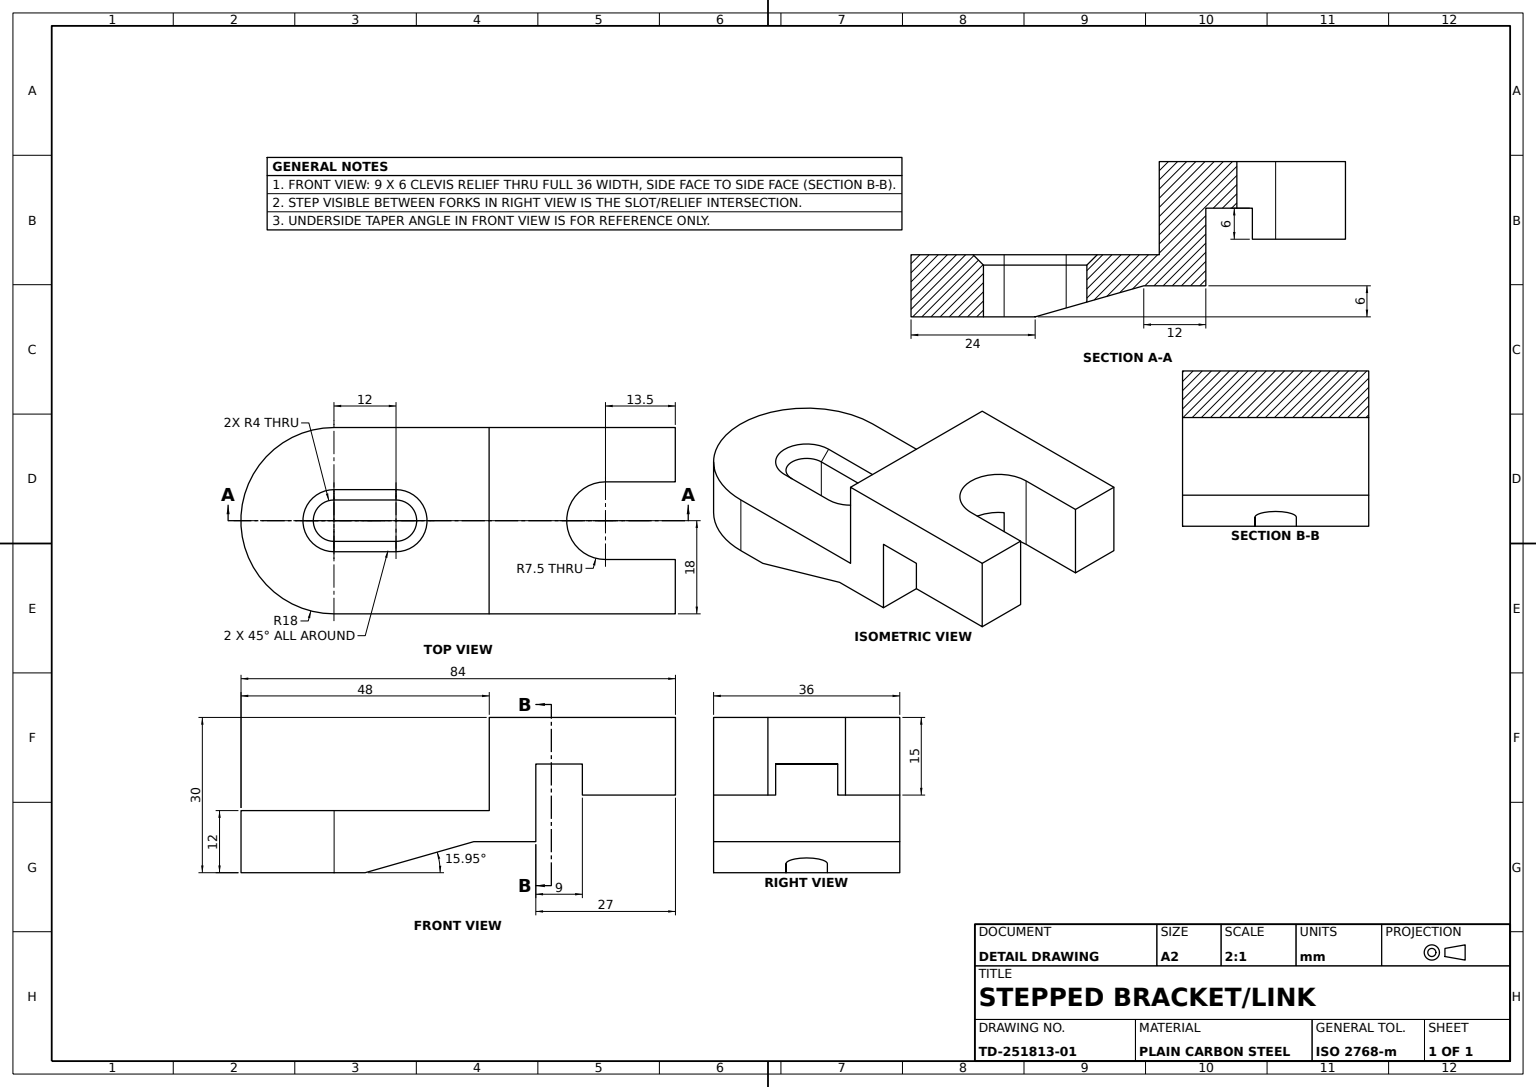
from build123d import *

# Parameters (mm, degrees)
HUB_SKETCH_R                = 18
HUB_36_DEPTH                = 12
ARM_START                   = -12
ARM_DEPTH                   = 12
HUB_SLOT_CHAMFER_45_DEPTH   = 2
HUB_SLOT_CHAMFER_45_DRAFT   = -45
HUB_SLOT_DEPTH              = 18
CLEVIS_BLOCK_DEPTH          = 36
CLEVIS_U_SLOT_SKETCH_W      = 13.5
CLEVIS_U_SLOT_SKETCH_H      = 15
CLEVIS_U_SLOT_DEPTH         = 90
BLOCK_STEP_CUT_DEPTH        = 60
BLOCK_STEP_CUT_DEPTH_BACK   = 147
BLOCK_STEP_CUT_SKETCH_W     = 9
BLOCK_STEP_CUT_SKETCH_H     = 21
ARM_TAPER_CUT_DEPTH         = 73
ARM_TAPER_CUT_DEPTH_BACK    = 190
ARM_TAPER_CUT_SKETCH_W      = 18
ARM_TAPER_CUT_SKETCH_H      = 15
BLOCK_RELIEF_CUT_DEPTH      = 190
BLOCK_RELIEF_CUT_DEPTH_BACK = 190


with BuildPart() as part:
    # Hub Sketch → Hub _36 (new body)
    with BuildSketch(Plane(origin=(0, 0, 0), x_dir=(1, 0, 0), z_dir=(0, 1, 0))):
        with Locations(Location((0, 0, 0), (0, 0, 270))):
            Circle(HUB_SKETCH_R)
    extrude(amount=HUB_36_DEPTH)

    # Arm Sketch → Arm (add)
    with BuildSketch(Plane(origin=(0, 12, 0), x_dir=(1, 0, 0), z_dir=(0, 1, 0)).offset(ARM_START)):
        with BuildLine():
            Line((30, 0), (18, 0))
            ThreePointArc((18, 0), (12.727922061, -12.727922061), (0, -18))
            Line((0, -18), (30, -18))
            Line((30, -18), (30, 0))
        make_face()
        with BuildLine():
            ThreePointArc((0, 18), (12.727922061, 12.727922061), (18, 0))
            Line((18, 0), (30, 0))
            Line((30, 0), (30, 18))
            Line((30, 18), (0, 18))
        make_face()
    extrude(amount=ARM_DEPTH)


with BuildPart() as hub_slot_chamfer_45_tool:
    # Hub Slot Chamfer Sketch → Hub Slot Chamfer 45 (with draft: the straight prism first)
    with BuildSketch(Plane(origin=(0, 12, 0), x_dir=(1, 0, 0), z_dir=(0, 1, 0))):
        with BuildLine():
            ThreePointArc((0, 6), (-6, 0), (0, -6))
            Line((0, -6), (12, -6))
            ThreePointArc((12, -6), (18, 0), (12, 6))
            Line((12, 6), (0, 6))
        make_face()
    extrude(amount=-HUB_SLOT_CHAMFER_45_DEPTH)
    # Hub Slot Chamfer 45: the draft: its side faces are tilted about the plane it starts from
    hub_slot_chamfer_45_sides = [hub_slot_chamfer_45_tool.faces().sort_by_distance(p)[0] for p in [
        (6, 11, -6),
        (-6, 11, 0),
        (6, 11, 6),
        (18, 11, 0),
    ]]
    draft(hub_slot_chamfer_45_sides, Plane(origin=(0, 12, 0), x_dir=(1, 0, 0), z_dir=(0, 1, 0)), HUB_SLOT_CHAMFER_45_DRAFT)


with BuildPart() as part_1:
    add(part.part)

    # Hub Slot Chamfer 45: cut by hub_slot_chamfer_45_tool
    add(hub_slot_chamfer_45_tool.part, mode=Mode.SUBTRACT)

    # Hub Slot Sketch → Hub Slot (cut)
    with BuildSketch(Plane(origin=(0, 10, 0), x_dir=(1, 0, 0), z_dir=(0, 1, 0))):
        with BuildLine():
            Line((12, 4), (0, 4))
            ThreePointArc((0, 4), (2.828427125, 2.828427125), (4, 0))
            ThreePointArc((4, 0), (2.828427125, -2.828427125), (0, -4))
            Line((0, -4), (12, -4))
            ThreePointArc((12, -4), (8, 0), (12, 4))
        make_face()
        with BuildLine():
            ThreePointArc((4, 0), (2.828427125, 2.828427125), (0, 4))
            ThreePointArc((0, 4), (-4, 0), (0, -4))
            ThreePointArc((0, -4), (2.828427125, -2.828427125), (4, 0))
        make_face()
        with BuildLine():
            ThreePointArc((16, 0), (14.828427125, 2.828427125), (12, 4))
            ThreePointArc((12, 4), (8, 0), (12, -4))
            ThreePointArc((12, -4), (14.828427125, -2.828427125), (16, 0))
        make_face()
    extrude(amount=-HUB_SLOT_DEPTH, mode=Mode.SUBTRACT)

    # Clevis Block Sketch → Clevis Block (add)
    with BuildSketch(Plane.XY.offset(18)):
        Polygon((30, 12), (30, 30), (66, 30), (66, 15), (66, 0), (30, 0), align=None)
    extrude(amount=-CLEVIS_BLOCK_DEPTH)

    # Clevis U-Slot Sketch → Clevis U-Slot (cut)
    with BuildSketch(Plane(origin=(0, 30, 0), x_dir=(1, 0, 0), z_dir=(0, 1, 0))):
        with BuildLine():
            Line((52.5, -7.5), (52.5, 7.5))
            ThreePointArc((52.5, 7.5), (45, 0), (52.5, -7.5))
        make_face()
        with Locations((59.25, 0)):
            Rectangle(CLEVIS_U_SLOT_SKETCH_W, CLEVIS_U_SLOT_SKETCH_H)
    extrude(amount=-CLEVIS_U_SLOT_DEPTH, mode=Mode.SUBTRACT)

    # Block Step Cut Sketch → Block Step Cut (cut, two sides: drawn at the far end of the back side and taken through both)
    with BuildSketch(Plane.XY.offset(18).offset(-BLOCK_STEP_CUT_DEPTH_BACK)):
        with Locations((43.5, 10.5)):
            Rectangle(BLOCK_STEP_CUT_SKETCH_W, BLOCK_STEP_CUT_SKETCH_H)
    extrude(amount=BLOCK_STEP_CUT_DEPTH + BLOCK_STEP_CUT_DEPTH_BACK, mode=Mode.SUBTRACT)

    # Arm Taper Cut Sketch → Arm Taper Cut (cut, two sides: drawn at the far end of the back side and taken through both)
    with BuildSketch(Plane.XY.offset(18).offset(-ARM_TAPER_CUT_DEPTH_BACK)):
        with Locations((57, 7.5)):
            Rectangle(ARM_TAPER_CUT_SKETCH_W, ARM_TAPER_CUT_SKETCH_H)
    extrude(amount=ARM_TAPER_CUT_DEPTH + ARM_TAPER_CUT_DEPTH_BACK, mode=Mode.SUBTRACT)

    # Block Relief Cut Sketch → Block Relief Cut (cut, two sides: drawn at the far end of the back side and taken through both)
    with BuildSketch(Plane.XY.offset(18).offset(-BLOCK_RELIEF_CUT_DEPTH_BACK)):
        Polygon((39, 0), (39, 6), (27, 6), (6, 0), align=None)
    extrude(amount=BLOCK_RELIEF_CUT_DEPTH + BLOCK_RELIEF_CUT_DEPTH_BACK, mode=Mode.SUBTRACT)


solid = part_1.part
